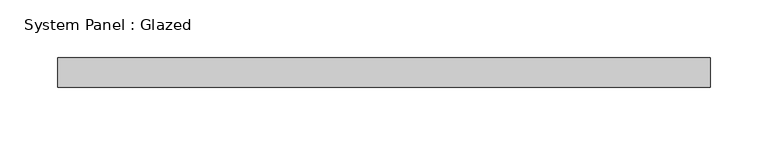
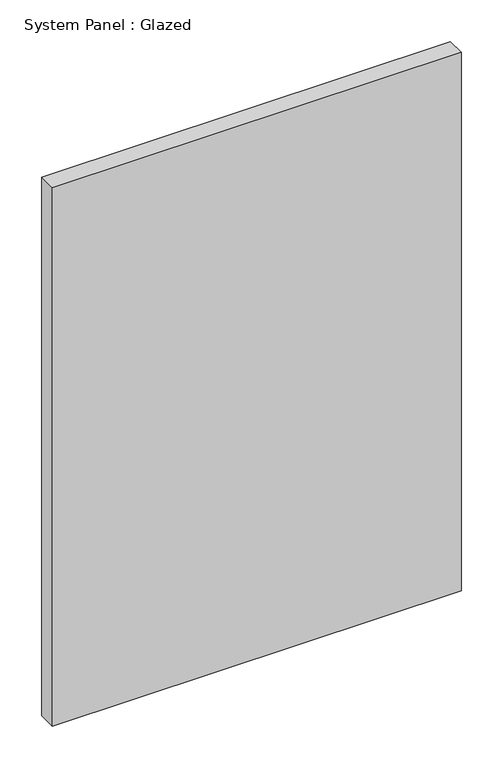
"""IFC4 building model written with IfcOpenShell, lengths in millimetres: plate geometry, System Panel : Glazed."""

from ifc_helpers import new_model, si_unit, origin, origin_with_axes, place, context, project, spatial, polyline, outline, extrude, source, transform, mapped, element, save


def system_panel_glazed_b4a8312c(model_context):
    return source(origin(), model_context, "Body", "SweptSolid", [
        extrude(outline(polyline([(282.575, -44.45), (-282.575, -44.45), (-282.575, -19.05), (282.575, -19.05), (282.575, -44.45)])), origin_with_axes(), (0.0, 0.0, 1.0), 787.4),
    ])


if __name__ == "__main__":
    model = new_model("IFC4")
    model_context = context("Model", 3, world=origin())
    ifc_project = project(units=[si_unit("LENGTHUNIT", "METRE", prefix="MILLI")], contexts=[model_context])
    site = spatial("IfcSite", under=ifc_project)
    building = spatial("IfcBuilding", under=site)
    placement = place(None, origin())
    system_panel_glazed_shape = system_panel_glazed_b4a8312c(model_context)
    element("IfcPlate", 1, ObjectType="System Panel : Glazed", at=placement, inside=building, context=model_context, shape_type="MappedRepresentation", body=[
        mapped(system_panel_glazed_shape, transform((0.0, 0.0, 0.0), x_axis=(1.0, 0.0, 0.0), y_axis=(0.0, 1.0, 0.0), z_axis=(0.0, 0.0, 1.0))),
    ])
    save(model, "model.ifc")

# Revit data of these elements
# Type "System Panel : Glazed"
#   Construction Type Id = "GSP4R"
#   Analytic Construction = "1/8 in Pilkington single glazing"
#   Visual Light Transmittance = 0.9
#   Solar Heat Gain Coefficient = 0.86
#   Heat Transfer Coefficient (U) = 1.18115 BTU/(h·ft²·°F)
#   Define Thermal Properties by = 1
# Element 1 (IfcPlate, "System Panel : Glazed")
#   Materials on its faces: "Glass"
# Materials
#   "Glass": class "Glass", colour RGB 0 128 192, transparency 0.75, Description = "Soda Lime Glass", Cost = 0
